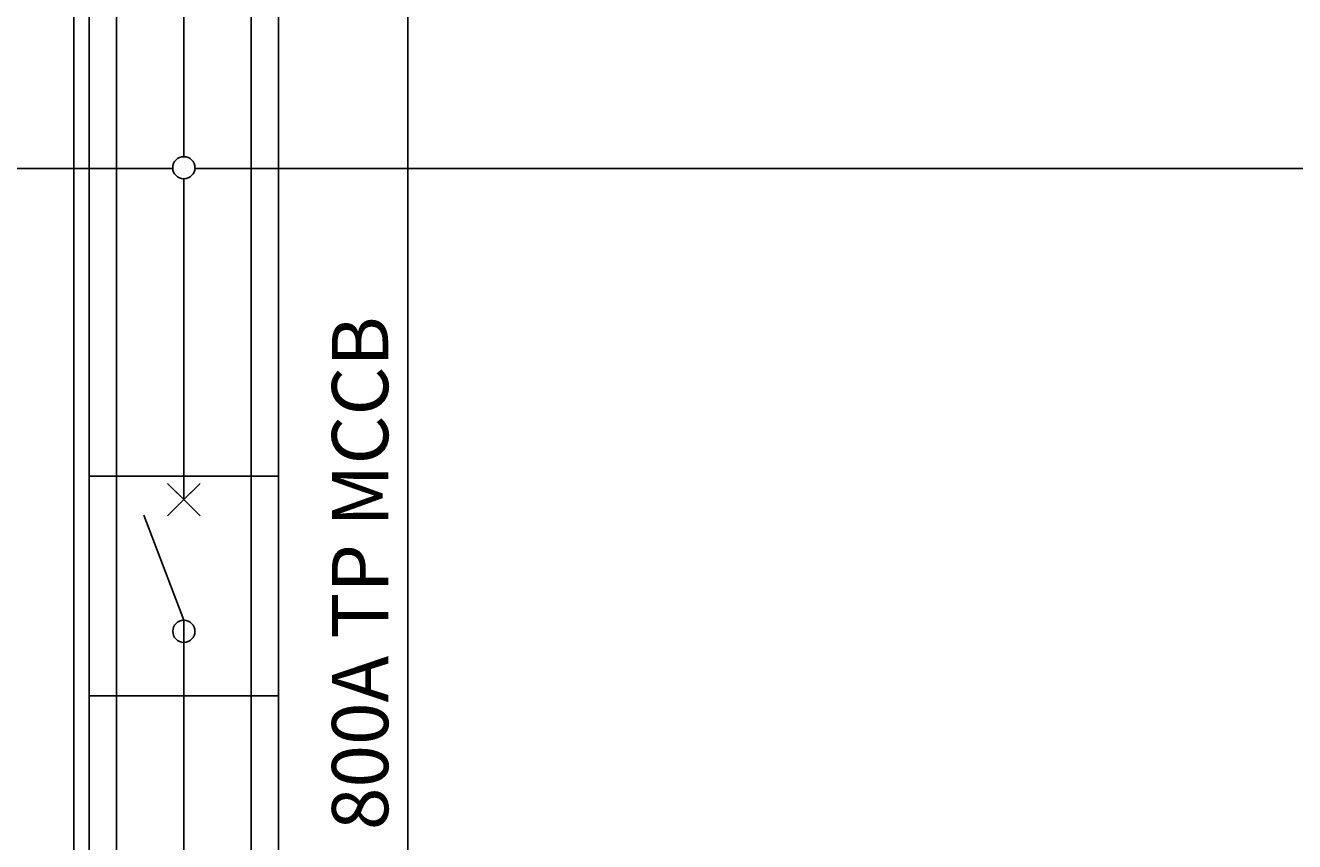
# Model space of a CAD drawing. Units: inches. Extents: x 412 to 584, y 208 to 437.
# Tile 8 of 28: x 494 to 539, y 233 to 262. Entities that reach past the tile are written whole.
import ezdxf

# ---------------------------------------------------------------- set-up
doc = ezdxf.new("R2010")
doc.units = ezdxf.units.IN
doc.header["$MEASUREMENT"] = 0
for name, color, linetype, lineweight in [('A-ANNO-DIMS', 2, 'Continuous', 18), ('E-ANNO-TEXT', 7, 'Continuous', 18), ('E-POWR-EQPM', 3, 'Continuous', 25)]:
    doc.layers.add(name, color=color, linetype=linetype, lineweight=lineweight)
doc.styles.get("Standard").update_dxf_attribs({"font": 'arial.ttf'})
doc.dimstyles.get("Standard").update_dxf_attribs({"dimtxt": 0.18, "dimasz": 0.18, "dimexe": 0.18, "dimexo": 0.0625, "dimgap": 0.09, "dimtad": 0, "dimtih": 1, "dimtoh": 1, "dimdec": 4, "dimzin": 0, "dimdsep": 46, "dimtxsty": 'Standard', "dimcen": 0.09, "dimadec": 0, "dimazin": 0, "dimtfac": 1, "dimtdec": 4, "dimtofl": 0, "dimtmove": 0, "dimatfit": 3, "dimfxl": 1, "dimtolj": 1, "dimtzin": 0, "dimarcsym": 0})

# ---------------------------------------------------------------- blocks, each defined once
blk = doc.blocks.new('*U3')
blk.add_line((-0.212, 0.212), (0.212, -0.212))
blk = doc.blocks.new('*U4')
at = {"color": 0, "linetype": 'ByBlock', "lineweight": -2, "transparency": 16777216}
for p, rotation in [((224.254, 56.203), 180), ((224.677, 56.203), 89.99999999999999), ((224.254, 55.78), 269.9999999999999)]:
    blk.add_blockref('*U3', p, dxfattribs=dict(at, rotation=rotation))
blk.add_blockref('*U3', (224.677, 55.78), dxfattribs=at)
blk = doc.blocks.new('*U7')
blk.add_line((-0.288, 0.288), (0.288, -0.288))
blk = doc.blocks.new('*U8')
at = {"color": 0, "linetype": 'ByBlock', "lineweight": -2, "transparency": 16777216}
for p, rotation in [((224.177, 56.28), 180), ((224.754, 56.28), 90), ((224.177, 55.703), 269.9999999999999)]:
    blk.add_blockref('*U7', p, dxfattribs=dict(at, rotation=rotation))
blk.add_blockref('*U7', (224.754, 55.703), dxfattribs=at)
blk = doc.blocks.new('MCCB-800A')
for q in [(1.94, 18.628), (3.361, 0)]:
    blk.add_line((3.361, 14.893), q)
blk.add_lwpolyline([(0, 20.016), (6.722, 20.016), (6.722, 12.209), (0, 12.209)], close=True)
blk.add_circle((3.361, 14.5), 0.393)
for name in ['*U8', '*U4']:
    blk.add_blockref(name, (-221.104, -36.809))
blk = doc.blocks.new('*D17')
at = {"layer": 'A-ANNO-DIMS', "color": 0, "lineweight": -2, "transparency": 16777216}
for p, q in [((497.715, 426.185), (583.674, 426.185)), ((583.494, 426.005), (583.494, 323.031)), ((583.494, 219.693), (583.494, 322.667)), ((550.198, 219.513), (583.674, 219.513))]:
    blk.add_line(p, q, dxfattribs=at)
at = {"layer": 'A-ANNO-DIMS', "color": 0, "transparency": 16777216}
for points in [[(583.464, 426.005), (583.524, 426.005), (583.494, 426.185)], [(583.464, 219.693), (583.524, 219.693), (583.494, 219.513)]]:
    blk.add_solid(points, dxfattribs=at)
at = {"layer": 'Defpoints', "color": 0, "transparency": 16777216}
for p in [(497.652, 426.185), (550.135, 219.513), (583.494, 219.513)]:
    blk.add_point(p, dxfattribs=at)
at = {"layer": 'A-ANNO-DIMS', "color": 0, "transparency": 16777216, "insert": (583.494, 322.849), "char_height": 0.18, "attachment_point": 5}
blk.add_mtext('\\A1;206.67', dxfattribs=at)
blk = doc.blocks.new('*D28')
at = {"layer": 'A-ANNO-DIMS', "color": 0, "lineweight": -2, "transparency": 16777216}
for p, q in [((450.562, 256.635), (450.562, 437.465)), ((450.742, 437.285), (502.724, 437.285)), ((555.616, 437.285), (503.634, 437.285)), ((555.796, 256.635), (555.796, 437.465))]:
    blk.add_line(p, q, dxfattribs=at)
at = {"layer": 'A-ANNO-DIMS', "color": 0, "transparency": 16777216}
for points in [[(450.742, 437.315), (450.742, 437.255), (450.562, 437.285)], [(555.616, 437.315), (555.616, 437.255), (555.796, 437.285)]]:
    blk.add_solid(points, dxfattribs=at)
at = {"layer": 'Defpoints', "color": 0, "transparency": 16777216}
for p in [(555.796, 437.285), (450.562, 256.573), (555.796, 256.573)]:
    blk.add_point(p, dxfattribs=at)
at = {"layer": 'A-ANNO-DIMS', "color": 0, "transparency": 16777216, "insert": (503.179, 437.285), "char_height": 0.18, "attachment_point": 5}
blk.add_mtext('\\A1;105.23', dxfattribs=at)
blk = doc.blocks.new('*D29')
at = {"layer": 'A-ANNO-DIMS', "color": 0, "lineweight": -2, "transparency": 16777216}
for p, q in [((495.927, 378.924), (495.927, 208.233)), ((502.649, 378.924), (502.649, 208.233)), ((496.107, 208.413), (498.895, 208.413)), ((502.469, 208.413), (499.681, 208.413))]:
    blk.add_line(p, q, dxfattribs=at)
at = {"layer": 'A-ANNO-DIMS', "color": 0, "transparency": 16777216}
for points in [[(496.107, 208.443), (496.107, 208.383), (495.927, 208.413)], [(502.469, 208.443), (502.469, 208.383), (502.649, 208.413)]]:
    blk.add_solid(points, dxfattribs=at)
at = {"layer": 'Defpoints', "color": 0, "transparency": 16777216}
for p in [(495.927, 378.987), (502.649, 378.987), (502.649, 208.413)]:
    blk.add_point(p, dxfattribs=at)
at = {"layer": 'A-ANNO-DIMS', "color": 0, "transparency": 16777216, "insert": (499.288, 208.413), "char_height": 0.18, "attachment_point": 5}
blk.add_mtext('\\A1;6.722', dxfattribs=at)
blk = doc.blocks.new('*D31')
at = {"layer": 'A-ANNO-DIMS', "color": 0, "lineweight": -2, "transparency": 16777216}
for p, q in [((495.375, 405.385), (495.375, 208.233)), ((507.254, 405.385), (507.254, 208.233)), ((495.555, 208.413), (500.929, 208.413)), ((507.074, 208.413), (501.7, 208.413))]:
    blk.add_line(p, q, dxfattribs=at)
at = {"layer": 'A-ANNO-DIMS', "color": 0, "transparency": 16777216}
for points in [[(495.555, 208.443), (495.555, 208.383), (495.375, 208.413)], [(507.074, 208.443), (507.074, 208.383), (507.254, 208.413)]]:
    blk.add_solid(points, dxfattribs=at)
at = {"layer": 'Defpoints', "color": 0, "transparency": 16777216}
for p in [(495.375, 405.448), (507.254, 405.448), (507.254, 208.413)]:
    blk.add_point(p, dxfattribs=at)
at = {"layer": 'A-ANNO-DIMS', "color": 0, "transparency": 16777216, "insert": (501.314, 208.413), "char_height": 0.18, "attachment_point": 5}
blk.add_mtext('\\A1;11.88', dxfattribs=at)
blk = doc.blocks.new('*D39')
at = {"layer": 'A-ANNO-DIMS', "color": 0, "lineweight": -2, "transparency": 16777216}
for p, q in [((496.891, 346.914), (496.891, 208.233)), ((501.685, 346.914), (501.685, 208.233)), ((497.071, 208.413), (498.891, 208.413)), ((501.505, 208.413), (499.685, 208.413))]:
    blk.add_line(p, q, dxfattribs=at)
at = {"layer": 'A-ANNO-DIMS', "color": 0, "transparency": 16777216}
for points in [[(497.071, 208.443), (497.071, 208.383), (496.891, 208.413)], [(501.505, 208.443), (501.505, 208.383), (501.685, 208.413)]]:
    blk.add_solid(points, dxfattribs=at)
at = {"layer": 'Defpoints', "color": 0, "transparency": 16777216}
for p in [(496.891, 346.977), (501.685, 346.977), (501.685, 208.413)]:
    blk.add_point(p, dxfattribs=at)
at = {"layer": 'A-ANNO-DIMS', "color": 0, "transparency": 16777216, "insert": (499.288, 208.413), "char_height": 0.18, "attachment_point": 5}
blk.add_mtext('\\A1;4.794', dxfattribs=at)

msp = doc.modelspace()

# ---------------------------------------------------------------- linework, layer by layer
at = {"layer": 'E-POWR-EQPM'}
for p, q in [((499.2878, 276.6357), (499.2878, 256.9861)), ((455.0375, 256.5729), (498.8949, 256.5729)), ((499.6808, 256.5729), (549.7416, 256.5729)), ((499.2878, 256.1992), (499.2878, 244.7899))]:
    msp.add_line(p, q, dxfattribs=at)
msp.add_circle((499.2878, 256.5926), 0.3935, dxfattribs=at)

# ---------------------------------------------------------------- block references
msp.add_blockref('MCCB-800A', (495.9268, 225.6077), dxfattribs=at)

# ---------------------------------------------------------------- texts
at = {"layer": 'E-ANNO-TEXT', "insert": (504.5509, 228.1355), "char_height": 2, "attachment_point": 1, "rotation": 90}
msp.add_mtext_dynamic_manual_height_columns('\\pxqc;800A TP MCCB', width=28.077497, gutter_width=1, heights=[9.1162], dxfattribs=at)

# ---------------------------------------------------------------- dimensions: what is measured, and where the dimension line sits
at = {"layer": 'A-ANNO-DIMS'}
for base, p1, p2, override, picture, middle in [((555.7959, 437.2847), (450.562, 256.5729), (555.7959, 256.5729), {"dimdec": 2, "dimlfac": 1, "dimrnd": 0, "dimzin": 0, "dimdsep": 46, "dimlunit": 2}, '*D28', (503.1789, 437.2847)), ((507.2538, 208.4133), (495.3746, 405.448), (507.2538, 405.448), {"dimdec": 2, "dimlfac": 1, "dimrnd": 0, "dimzin": 0, "dimdsep": 46, "dimlunit": 2}, '*D31', (501.3142, 208.4133)), ((502.6489, 208.4133), (495.9268, 378.9867), (502.6489, 378.9867), {"dimdec": 3, "dimlfac": 1, "dimrnd": 0, "dimzin": 0, "dimdsep": 46, "dimlunit": 2}, '*D29', (499.2878, 208.4133)), ((501.6846, 208.4133), (496.891, 346.9765), (501.6846, 346.9765), {"dimdec": 3, "dimlfac": 1, "dimrnd": 0, "dimzin": 0, "dimdsep": 46, "dimlunit": 2}, '*D39', (499.2878, 208.4133))]:
    dim = msp.add_linear_dim(base=base, p1=p1, p2=p2, dimstyle='Standard', override=override, dxfattribs=at)
    dim.commit()
    dim.dimension.update_dxf_attribs({"geometry": picture, "text_midpoint": middle})
dim = msp.add_linear_dim(base=(583.4937, 219.5133), p1=(497.6523, 426.1847), p2=(550.1351, 219.5133), angle=90, dimstyle='Standard', override={"dimdec": 2, "dimlfac": 1, "dimrnd": 0, "dimzin": 0, "dimdsep": 46, "dimlunit": 2}, dxfattribs=at)
dim.commit()
dim.dimension.update_dxf_attribs({"geometry": '*D17', "text_midpoint": (583.4937, 322.849)})

doc.saveas('drawing.dxf')
